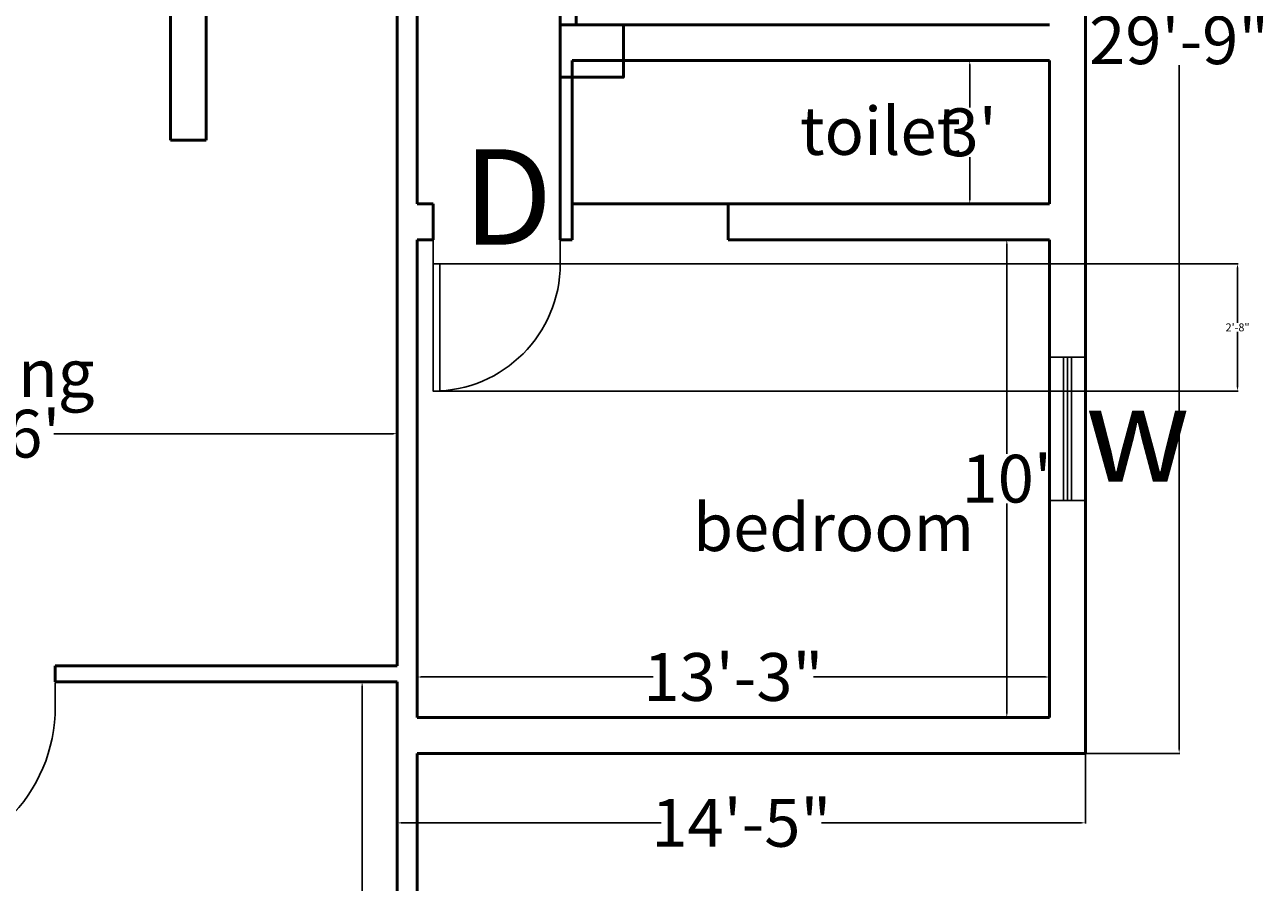
# Model space of a CAD drawing. Units: inches. Extents: x 409 to 7572, y 7 to 725.
# Tile 19 of 38: x 3250 to 3562, y 283 to 499. Entities that reach past the tile are written whole.
import ezdxf

# ---------------------------------------------------------------- set-up
doc = ezdxf.new("R2010")
doc.units = ezdxf.units.IN
doc.header["$MEASUREMENT"] = 0
for name, color, linetype, lineweight in [('A-ANNO-DIMS', 2, 'Continuous', 18), ('A-ANNO-SYMB', 3, 'Continuous', 25), ('A-AREA-IDEN', 7, 'Continuous', 25), ('A-DOOR', 3, 'Continuous', 25), ('A-GLAZ', 4, 'Continuous', 25), ('A-WALL', 7, 'Continuous', 50)]:
    doc.layers.add(name, color=color, linetype=linetype, lineweight=lineweight)
doc.styles.get("Standard").update_dxf_attribs({"font": 'arial.ttf'})
doc.dimstyles.get("Standard").update_dxf_attribs({"dimtxt": 2, "dimasz": 1, "dimexe": 0.18, "dimexo": 0.0625, "dimgap": 0.09, "dimtad": 0, "dimtih": 1, "dimtoh": 1, "dimdec": 0, "dimzin": 0, "dimdsep": 46, "dimlunit": 3, "dimtxsty": 'Standard', "dimcen": 0.09, "dimadec": 0, "dimazin": 0, "dimtfac": 1, "dimtdec": 0, "dimtofl": 0, "dimtmove": 0, "dimatfit": 3, "dimfxl": 1, "dimtolj": 1, "dimtzin": 0, "dimarcsym": 0})

# ---------------------------------------------------------------- blocks, each defined once
blk = doc.blocks.new('*U5')
for p, q in [((0, 0), (0, 6)), ((40, 0), (40, 6))]:
    blk.add_line(p, q)
blk.add_lwpolyline([(0, 0), (0, -40), (1.75, -40), (1.75, 0)], close=True)
blk.add_arc((0, 0), 40, 270, 0)
blk = doc.blocks.new('*U7')
for p, q in [((0, 0), (0, 6)), ((32, 0), (32, 6))]:
    blk.add_line(p, q)
blk.add_lwpolyline([(0, 0), (0, -32), (1.75, -32), (1.75, 0)], close=True)
blk.add_arc((0, 0), 32, 270, 0)
blk = doc.blocks.new('*D75')
at = {"layer": 'A-ANNO-DIMS', "color": 0, "lineweight": -2, "transparency": 16777216}
for p, q in [((3508.04, 444.53), (3497.15, 444.53)), ((3497.33, 443.53), (3497.33, 390.75)), ((3497.33, 325.53), (3497.33, 378.31)), ((3508.04, 324.53), (3497.15, 324.53))]:
    blk.add_line(p, q, dxfattribs=at)
at = {"layer": 'A-ANNO-DIMS', "color": 0, "transparency": 16777216}
for points in [[(3497.17, 443.53), (3497.5, 443.53), (3497.33, 444.53)], [(3497.17, 325.53), (3497.5, 325.53), (3497.33, 324.53)]]:
    blk.add_solid(points, dxfattribs=at)
at = {"layer": 'DEFPOINTS', "color": 0, "transparency": 16777216}
for p in [(3497.33, 444.53), (3508.1, 444.53), (3508.1, 324.53)]:
    blk.add_point(p, dxfattribs=at)
at = {"layer": 'A-ANNO-DIMS', "color": 0, "transparency": 16777216, "insert": (3497.33, 384.53), "char_height": 2, "attachment_point": 5}
blk.add_mtext("\\A1;{\\H6x;10'}", dxfattribs=at)
blk = doc.blocks.new('*D66')
at = {"layer": 'A-ANNO-DIMS', "color": 0, "lineweight": -2, "transparency": 16777216}
for p, q in [((3349.1, 324.59), (3349.1, 334.9)), ((3350.1, 334.72), (3408.46, 334.72)), ((3507.1, 334.72), (3448.73, 334.72)), ((3508.1, 324.59), (3508.1, 334.9))]:
    blk.add_line(p, q, dxfattribs=at)
at = {"layer": 'A-ANNO-DIMS', "color": 0, "transparency": 16777216}
for points in [[(3350.1, 334.88), (3350.1, 334.55), (3349.1, 334.72)], [(3507.1, 334.88), (3507.1, 334.55), (3508.1, 334.72)]]:
    blk.add_solid(points, dxfattribs=at)
at = {"layer": 'DEFPOINTS', "color": 0, "transparency": 16777216}
for p in [(3349.1, 334.72), (3349.1, 324.53), (3508.1, 324.53)]:
    blk.add_point(p, dxfattribs=at)
at = {"layer": 'A-ANNO-DIMS', "color": 0, "transparency": 16777216, "insert": (3428.6, 334.72), "char_height": 2, "attachment_point": 5}
blk.add_mtext('\\A1;{\\H6x;13\'-3"}', dxfattribs=at)
blk = doc.blocks.new('*D67')
at = {"layer": 'A-ANNO-DIMS', "color": 0, "lineweight": -2, "transparency": 16777216}
for p, q in [((3344.04, 333.53), (3335.1, 333.53)), ((3335.28, 332.53), (3335.28, 255.65)), ((3335.28, 166.53), (3335.28, 243.42)), ((3344.04, 165.53), (3335.1, 165.53))]:
    blk.add_line(p, q, dxfattribs=at)
at = {"layer": 'A-ANNO-DIMS', "color": 0, "transparency": 16777216}
for points in [[(3335.12, 332.53), (3335.45, 332.53), (3335.28, 333.53)], [(3335.12, 166.53), (3335.45, 166.53), (3335.28, 165.53)]]:
    blk.add_solid(points, dxfattribs=at)
at = {"layer": 'DEFPOINTS', "color": 0, "transparency": 16777216}
for p in [(3344.1, 333.53), (3335.28, 165.53), (3344.1, 165.53)]:
    blk.add_point(p, dxfattribs=at)
at = {"layer": 'A-ANNO-DIMS', "color": 0, "transparency": 16777216, "insert": (3335.28, 249.53), "char_height": 2, "attachment_point": 5}
blk.add_mtext("\\A1;{\\H6x;14'}", dxfattribs=at)
blk = doc.blocks.new('*D80')
at = {"layer": 'A-ANNO-DIMS', "color": 0, "lineweight": -2, "transparency": 16777216}
for p, q in [((3152.1, 403.47), (3152.1, 395.65)), ((3344.1, 403.47), (3344.1, 395.65)), ((3153.1, 395.83), (3238.39, 395.83)), ((3343.1, 395.83), (3257.81, 395.83))]:
    blk.add_line(p, q, dxfattribs=at)
at = {"layer": 'A-ANNO-DIMS', "color": 0, "transparency": 16777216}
for points in [[(3153.1, 396), (3153.1, 395.66), (3152.1, 395.83)], [(3343.1, 396), (3343.1, 395.66), (3344.1, 395.83)]]:
    blk.add_solid(points, dxfattribs=at)
at = {"layer": 'DEFPOINTS', "color": 0, "transparency": 16777216}
for p in [(3152.1, 403.53), (3344.1, 403.53), (3344.1, 395.83)]:
    blk.add_point(p, dxfattribs=at)
at = {"layer": 'A-ANNO-DIMS', "color": 0, "transparency": 16777216, "insert": (3248.1, 395.83), "char_height": 2, "attachment_point": 5}
blk.add_mtext("\\A1;{\\H6x;16'}", dxfattribs=at)
blk = doc.blocks.new('*D88')
at = {"layer": 'A-ANNO-DIMS', "color": 0, "lineweight": -2, "transparency": 16777216}
for p, q in [((3508.04, 489.53), (3487.84, 489.53)), ((3488.02, 488.53), (3488.02, 477.75)), ((3488.02, 454.53), (3488.02, 465.31)), ((3508.04, 453.53), (3487.84, 453.53))]:
    blk.add_line(p, q, dxfattribs=at)
at = {"layer": 'A-ANNO-DIMS', "color": 0, "transparency": 16777216}
for points in [[(3487.86, 488.53), (3488.19, 488.53), (3488.02, 489.53)], [(3487.86, 454.53), (3488.19, 454.53), (3488.02, 453.53)]]:
    blk.add_solid(points, dxfattribs=at)
at = {"layer": 'DEFPOINTS', "color": 0, "transparency": 16777216}
for p in [(3508.1, 489.53), (3488.02, 453.53), (3508.1, 453.53)]:
    blk.add_point(p, dxfattribs=at)
at = {"layer": 'A-ANNO-DIMS', "color": 0, "transparency": 16777216, "insert": (3488.02, 471.53), "char_height": 2, "attachment_point": 5}
blk.add_mtext("\\A1;{\\H6x;3'}", dxfattribs=at)
blk = doc.blocks.new('*D92')
at = {"layer": 'A-ANNO-DIMS', "color": 0, "lineweight": -2, "transparency": 16777216}
for p, q in [((3517.16, 672.53), (3540.84, 672.53)), ((3540.66, 671.53), (3540.66, 500.86)), ((3540.66, 316.53), (3540.66, 488.43)), ((3517.16, 315.53), (3540.84, 315.53))]:
    blk.add_line(p, q, dxfattribs=at)
at = {"layer": 'A-ANNO-DIMS', "color": 0, "transparency": 16777216}
for points in [[(3540.5, 671.53), (3540.83, 671.53), (3540.66, 672.53)], [(3540.5, 316.53), (3540.83, 316.53), (3540.66, 315.53)]]:
    blk.add_solid(points, dxfattribs=at)
at = {"layer": 'DEFPOINTS', "color": 0, "transparency": 16777216}
for p in [(3517.1, 672.53), (3540.66, 672.53), (3517.1, 315.53)]:
    blk.add_point(p, dxfattribs=at)
at = {"layer": 'A-ANNO-DIMS', "color": 0, "transparency": 16777216, "insert": (3540.66, 494.65), "char_height": 2, "attachment_point": 5}
blk.add_mtext('\\A1;{\\H6x;29\'-9"}', dxfattribs=at)
blk = doc.blocks.new('*D91')
at = {"layer": 'A-ANNO-DIMS', "color": 0, "lineweight": -2, "transparency": 16777216}
for p, q in [((3344.1, 315.37), (3344.1, 297.9)), ((3517.1, 315.37), (3517.1, 297.9)), ((3345.1, 298.08), (3410.46, 298.08)), ((3516.1, 298.08), (3450.73, 298.08))]:
    blk.add_line(p, q, dxfattribs=at)
at = {"layer": 'A-ANNO-DIMS', "color": 0, "transparency": 16777216}
for points in [[(3345.1, 298.25), (3345.1, 297.92), (3344.1, 298.08)], [(3516.1, 298.25), (3516.1, 297.92), (3517.1, 298.08)]]:
    blk.add_solid(points, dxfattribs=at)
at = {"layer": 'DEFPOINTS', "color": 0, "transparency": 16777216}
for p in [(3344.1, 315.43), (3517.1, 315.43), (3517.1, 298.08)]:
    blk.add_point(p, dxfattribs=at)
at = {"layer": 'A-ANNO-DIMS', "color": 0, "transparency": 16777216, "insert": (3430.6, 298.08), "char_height": 2, "attachment_point": 5}
blk.add_mtext('\\A1;{\\H6x;14\'-5"}', dxfattribs=at)
blk = doc.blocks.new('WIN-36')
for p, q in [((1699.82, 514.65), (1699.82, 478.65)), ((1700.82, 514.65), (1700.82, 478.65)), ((1701.82, 514.65), (1701.82, 478.65))]:
    blk.add_line(p, q)
blk.add_lwpolyline([(1705.32, 514.65), (1705.32, 478.65), (1696.32, 478.65), (1696.32, 514.65)], close=True)
blk = doc.blocks.new('*D186')
at = {"layer": 'A-ANNO-DIMS', "color": 0, "lineweight": -2, "transparency": 16777216}
for p, q in [((3353.16, 438.53), (3555.53, 438.53)), ((3555.35, 437.53), (3555.35, 423.64)), ((3555.35, 407.53), (3555.35, 421.42)), ((3353.16, 406.53), (3555.53, 406.53))]:
    blk.add_line(p, q, dxfattribs=at)
at = {"layer": 'A-ANNO-DIMS', "color": 0, "transparency": 16777216}
for points in [[(3555.18, 437.53), (3555.51, 437.53), (3555.35, 438.53)], [(3555.18, 407.53), (3555.51, 407.53), (3555.35, 406.53)]]:
    blk.add_solid(points, dxfattribs=at)
at = {"layer": 'DEFPOINTS', "color": 0, "transparency": 16777216}
for p in [(3353.1, 438.53), (3353.1, 406.53), (3555.35, 406.53)]:
    blk.add_point(p, dxfattribs=at)
at = {"layer": 'A-ANNO-DIMS', "color": 0, "transparency": 16777216, "insert": (3555.35, 422.53), "char_height": 2, "attachment_point": 5}
blk.add_mtext('\\A1;2\'-8"', dxfattribs=at)

msp = doc.modelspace()

# ---------------------------------------------------------------- linework, layer by layer
at = {"layer": 'A-WALL'}
for p, q in [((3517.1, 315.53), (3517.1, 672.53)), ((3349.1, 534.53), (3349.1, 453.53)), ((3296.1, 525.53), (3296.1, 469.53)), ((3344.1, 525.53), (3344.1, 337.53)), ((3385.1, 498.53), (3385.1, 503.53)), ((3389.1, 503.53), (3389.1, 498.53)), ((3508.1, 498.53), (3385.1, 498.53)), ((3385.1, 498.53), (3385.1, 444.53)), ((3344.1, 489.53), (3344.1, 337.53)), ((3508.1, 489.53), (3388.1, 489.53)), ((3388.1, 489.53), (3388.1, 444.53)), ((3508.1, 453.53), (3508.1, 489.53)), ((3287.1, 469.53), (3296.1, 469.53)), ((3353.1, 453.53), (3349.1, 453.53)), ((3353.1, 453.53), (3353.1, 444.53)), ((3508.1, 453.53), (3388.1, 453.53)), ((3427.29, 453.53), (3427.29, 444.53)), ((3353.1, 444.53), (3349.1, 444.53)), ((3349.1, 444.53), (3349.1, 324.53)), ((3388.1, 444.53), (3385.1, 444.53)), ((3388.1, 444.53), (3385.1, 444.53)), ((3508.1, 444.53), (3427.29, 444.53)), ((3508.1, 324.53), (3508.1, 444.53)), ((3258.16, 337.53), (3344.1, 337.53)), ((3258.16, 337.53), (3258.16, 333.53)), ((3258.16, 333.53), (3344.1, 333.53)), ((3344.1, 333.53), (3344.1, 165.53)), ((3344.1, 333.53), (3344.1, 165.53)), ((3508.1, 324.53), (3349.1, 324.53)), ((3517.1, 315.53), (3349.1, 315.53)), ((3349.1, 315.53), (3349.1, 165.53))]:
    msp.add_line(p, q, dxfattribs=at)
msp.add_lwpolyline([(3287.1, 594.53), (3287.1, 525.53), (3287.1, 469.53)], dxfattribs=at)
msp.add_lwpolyline([(3385.1, 498.53), (3400.96, 498.53), (3400.96, 485.36), (3385.1, 485.36)], close=True, dxfattribs=at)

# ---------------------------------------------------------------- block references
at = {"layer": 'A-DOOR'}
for name, p in [('*U7', (3353.1, 438.53)), ('*U5', (3218.16, 327.37))]:
    msp.add_blockref(name, p, dxfattribs=at)
at = {"layer": 'A-GLAZ'}
msp.add_blockref('WIN-36', (1811.78, -99.57), dxfattribs=at)

# ---------------------------------------------------------------- texts
at = {"layer": 'A-ANNO-SYMB', "char_height": 24, "attachment_point": 1}
for s, width, insert in [('D', 19.1972, (3360.6, 467.28)), ('w', 18.2582, (3517.1, 407.79))]:
    msp.add_mtext_dynamic_manual_height_columns(s, width=width, gutter_width=1, heights=[0], dxfattribs=dict(at, insert=insert))
at = {"layer": 'A-AREA-IDEN', "char_height": 12, "attachment_point": 1}
for s, width, insert in [('toilet', 49.2946, (3445.35, 477.86)), ('Dining ', 67.5069, (3218.53, 417.03)), ('bedroom', 40.9017, (3418.43, 378.34))]:
    msp.add_mtext_dynamic_manual_height_columns(s, width=width, gutter_width=1, heights=[0], dxfattribs=dict(at, insert=insert))

# ---------------------------------------------------------------- dimensions: what is measured, and where the dimension line sits
at = {"layer": 'A-ANNO-DIMS'}
dim = msp.add_linear_dim(base=(3540.66, 672.53), p1=(3517.1, 315.53), p2=(3517.1, 672.53), angle=90, text='{\\H6x;<>}', dimstyle='Standard', override={"dimclrd": 0, "dimclre": 0, "dimclrt": 0}, dxfattribs=at)
dim.commit()
dim.dimension.update_dxf_attribs({"geometry": '*D92', "text_midpoint": (3540.66, 494.65), "dimtype": 160})
for base, p1, p2, picture, middle in [((3488.02, 453.53), (3508.1, 489.53), (3508.1, 453.53), '*D88', (3488.02, 471.53)), ((3497.33, 444.53), (3508.1, 324.53), (3508.1, 444.53), '*D75', (3497.33, 384.53)), ((3335.28, 165.53), (3344.1, 333.53), (3344.1, 165.53), '*D67', (3335.28, 249.53))]:
    dim = msp.add_linear_dim(base=base, p1=p1, p2=p2, angle=90, text='{\\H6x;<>}', dimstyle='Standard', override={"dimclrd": 0, "dimclre": 0, "dimclrt": 0}, dxfattribs=at)
    dim.commit()
    dim.dimension.update_dxf_attribs({"geometry": picture, "text_midpoint": middle})
dim = msp.add_linear_dim(base=(3555.35, 406.53), p1=(3353.1, 438.53), p2=(3353.1, 406.53), angle=90, dimstyle='Standard', override={"dimdec": 1, "dimlfac": 1, "dimrnd": 0, "dimzin": 1, "dimdsep": 46, "dimlunit": 4, "dimfrac": 2}, dxfattribs=at)
dim.commit()
dim.dimension.update_dxf_attribs({"geometry": '*D186', "text_midpoint": (3555.35, 422.53)})
dim = msp.add_linear_dim(base=(3344.1, 395.83), p1=(3152.1, 403.53), p2=(3344.1, 403.53), text='{\\H6x;<>}', dimstyle='Standard', override={"dimclrd": 0, "dimclre": 0, "dimclrt": 0}, dxfattribs=at)
dim.commit()
dim.dimension.update_dxf_attribs({"geometry": '*D80', "text_midpoint": (3248.1, 395.83), "dimtype": 160})
for base, p1, p2, picture, middle in [((3349.1, 334.72), (3508.1, 324.53), (3349.1, 324.53), '*D66', (3428.6, 334.72)), ((3517.1, 298.08), (3344.1, 315.43), (3517.1, 315.43), '*D91', (3430.6, 298.08))]:
    dim = msp.add_linear_dim(base=base, p1=p1, p2=p2, text='{\\H6x;<>}', dimstyle='Standard', override={"dimclrd": 0, "dimclre": 0, "dimclrt": 0}, dxfattribs=at)
    dim.commit()
    dim.dimension.update_dxf_attribs({"geometry": picture, "text_midpoint": middle})

doc.saveas('drawing.dxf')
